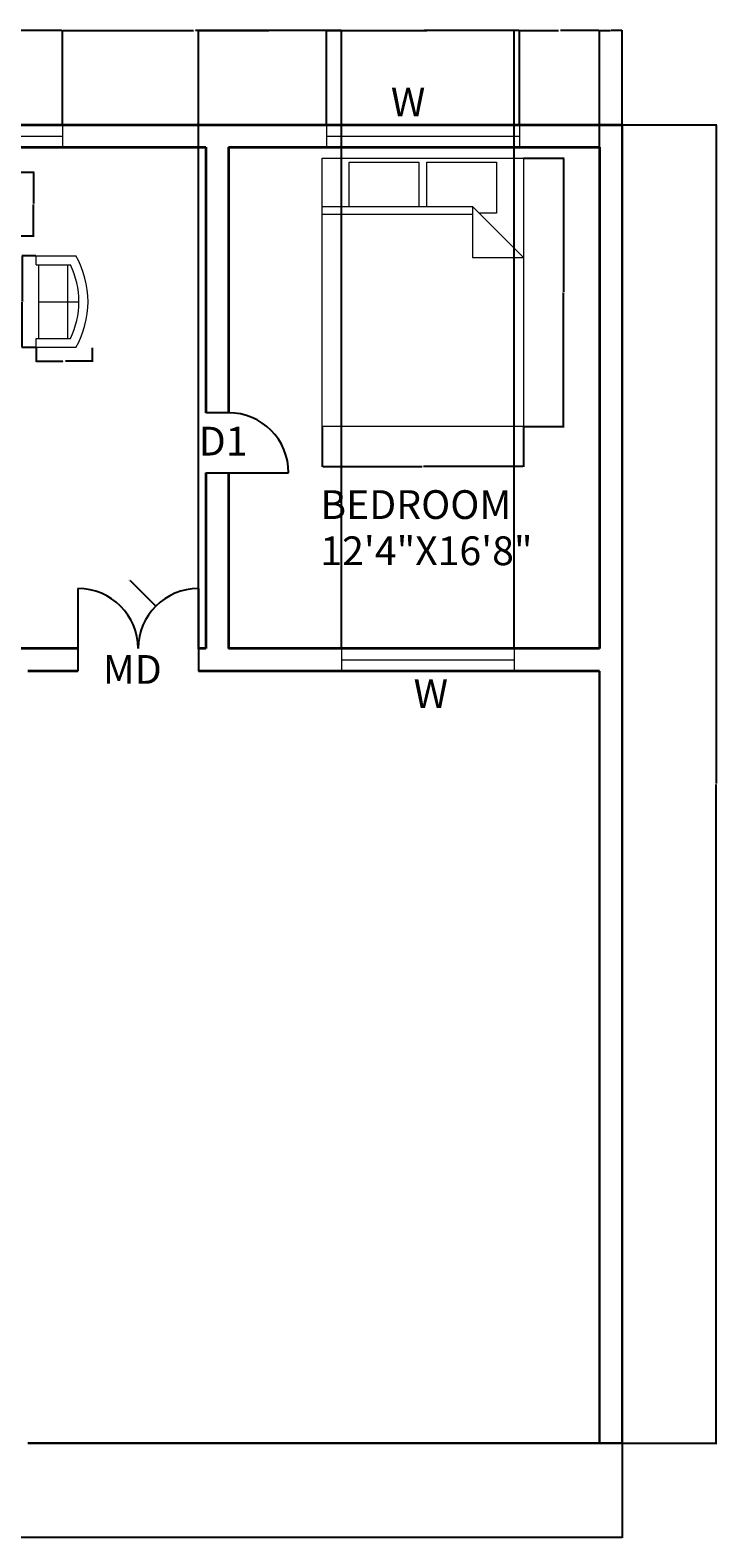
# Model space of a CAD drawing. Units: feet. Extents: x 1889 to 2708, y 1752 to 2375.
# Tile 5 of 5: x 2434 to 2708, y 1774 to 2375. Entities that reach past the tile are written whole.
import ezdxf

# ---------------------------------------------------------------- set-up
doc = ezdxf.new("R2010")
doc.units = ezdxf.units.FT
for name, color, linetype, lineweight in [('A-ANNO-DIMS', 2, 'Continuous', 18), ('A-ANNO-TEXT', 7, 'Continuous', 18), ('A-AREA-IDEN', 7, 'Continuous', 18), ('A-DOOR', 3, 'Continuous', 25), ('A-FURN', 8, 'Continuous', 18), ('A-GLAZ', 4, 'Continuous', 18), ('A-WALL', 7, 'Continuous', 35), ('C-PROP', 7, 'Continuous', 30)]:
    doc.layers.add(name, color=color, linetype=linetype, lineweight=lineweight)
doc.styles.get("Standard").update_dxf_attribs({"font": 'arial.ttf'})
doc.dimstyles.get("Standard").update_dxf_attribs({"dimtxt": 0.18, "dimasz": 0.18, "dimexe": 0.18, "dimexo": 0.0625, "dimgap": 0.09, "dimtad": 0, "dimtih": 1, "dimtoh": 1, "dimdec": 4, "dimzin": 0, "dimdsep": 46, "dimtxsty": 'Standard', "dimcen": 0.09, "dimadec": 0, "dimazin": 0, "dimtfac": 1, "dimtdec": 4, "dimtofl": 0, "dimtmove": 0, "dimatfit": 3, "dimfxl": 1, "dimtolj": 1, "dimtzin": 0, "dimarcsym": 0})

# ---------------------------------------------------------------- blocks, each defined once
blk = doc.blocks.new('Sofa - Roundback Loveseat 5 ft.')
for p, q in [((0, -32.44198), (0, -5.99998)), ((-24, -33.99998), (-24, -11.46958)), ((-23.9998, -13.38178), (23.99986, -13.38178)), ((24.00004, -33.99998), (24.00004, -11.46958)), ((-24, -32.44198), (24.00004, -32.44198))]:
    blk.add_line(p, q)
for points in [[(-24, -33.99998), (-30, -33.99998), (-30, -7.99998)], [(30.00004, -7.99998), (30.00004, -33.99998), (24.00004, -33.99998)]]:
    blk.add_lwpolyline(points)
for centre, radius, start, end in [((0, -60.24998), 60.24998, 60.13715, 119.8628), ((0, -61.38438), 55.38444, 64.32083, 115.6792)]:
    blk.add_arc(centre, radius, start, end)
blk = doc.blocks.new('Bed - Queen')
for p, q in [((0, -80.00003), (0, 0)), ((0, 0), (59.99999, 0)), ((59.99999, 0), (59.99999, -80.00003)), ((7.99999, -1.2), (28.79998, -1.2)), ((7.99999, -14.4), (7.99999, -1.2)), ((28.79998, -1.2), (28.79998, -14.4)), ((31.19999, -1.2), (51.99999, -1.2)), ((31.19999, -14.4), (31.19999, -1.2)), ((51.99999, -1.2), (51.99999, -16.4)), ((0, -14.4), (44.8, -14.4)), ((44.8, -16.8), (0, -16.8)), ((59.99999, -29.6), (44.8, -14.4)), ((44.8, -14.4), (44.8, -29.6)), ((51.99999, -16.4), (46.79936, -16.4)), ((44.8, -29.6), (59.99999, -29.6)), ((59.99999, -80.00003), (0, -80.00003))]:
    blk.add_line(p, q)
blk = doc.blocks.new('*D21')
at = {"layer": 'A-ANNO-DIMS', "color": 0, "lineweight": -2, "transparency": 16777216}
for p, q in [((2630.52, 2324.2), (2646.68, 2324.2)), ((2646.5, 2324.02), (2646.5, 2270.92)), ((2646.5, 2217.46), (2646.5, 2270.56)), ((2630.52, 2217.28), (2646.68, 2217.28))]:
    blk.add_line(p, q, dxfattribs=at)
at = {"layer": 'A-ANNO-DIMS', "color": 0, "transparency": 16777216}
for points in [[(2646.47, 2324.02), (2646.53, 2324.02), (2646.5, 2324.2)], [(2646.47, 2217.46), (2646.53, 2217.46), (2646.5, 2217.28)]]:
    blk.add_solid(points, dxfattribs=at)
at = {"layer": 'Defpoints', "color": 0, "transparency": 16777216}
for p in [(2630.46, 2324.2), (2646.5, 2324.2), (2630.46, 2217.28)]:
    blk.add_point(p, dxfattribs=at)
at = {"layer": 'A-ANNO-DIMS', "color": 0, "transparency": 16777216, "insert": (2646.5, 2270.74), "char_height": 0.18, "attachment_point": 5}
blk.add_mtext('\\A1;BED 107', dxfattribs=at)
blk = doc.blocks.new('*D22')
at = {"layer": 'A-ANNO-DIMS', "color": 0, "lineweight": -2, "transparency": 16777216}
for p, q in [((2550.26, 2217.22), (2550.26, 2201.06)), ((2630.46, 2217.22), (2630.46, 2201.06)), ((2550.44, 2201.24), (2590.14, 2201.24)), ((2630.28, 2201.24), (2590.58, 2201.24))]:
    blk.add_line(p, q, dxfattribs=at)
at = {"layer": 'A-ANNO-DIMS', "color": 0, "transparency": 16777216}
for points in [[(2550.44, 2201.27), (2550.44, 2201.21), (2550.26, 2201.24)], [(2630.28, 2201.27), (2630.28, 2201.21), (2630.46, 2201.24)]]:
    blk.add_solid(points, dxfattribs=at)
at = {"layer": 'Defpoints', "color": 0, "transparency": 16777216}
for p in [(2550.26, 2217.28), (2630.46, 2217.28), (2630.46, 2201.24)]:
    blk.add_point(p, dxfattribs=at)
at = {"layer": 'A-ANNO-DIMS', "color": 0, "transparency": 16777216, "insert": (2590.36, 2201.24), "char_height": 0.18, "attachment_point": 5}
blk.add_mtext('\\A1;80', dxfattribs=at)
blk = doc.blocks.new('*D24')
at = {"layer": 'A-ANNO-DIMS', "color": 0, "lineweight": -2, "transparency": 16777216}
for p, q in [((2426.47, 2318.69), (2435.33, 2318.69)), ((2435.15, 2318.51), (2435.15, 2306.15)), ((2435.15, 2293.42), (2435.15, 2305.78)), ((2426.47, 2293.24), (2435.33, 2293.24))]:
    blk.add_line(p, q, dxfattribs=at)
at = {"layer": 'A-ANNO-DIMS', "color": 0, "transparency": 16777216}
for points in [[(2435.12, 2318.51), (2435.18, 2318.51), (2435.15, 2318.69)], [(2435.12, 2293.42), (2435.18, 2293.42), (2435.15, 2293.24)]]:
    blk.add_solid(points, dxfattribs=at)
at = {"layer": 'Defpoints', "color": 0, "transparency": 16777216}
for p in [(2426.4, 2318.69), (2435.15, 2318.69), (2426.4, 2293.24)]:
    blk.add_point(p, dxfattribs=at)
at = {"layer": 'A-ANNO-DIMS', "color": 0, "transparency": 16777216, "insert": (2435.15, 2305.97), "char_height": 0.18, "attachment_point": 5}
blk.add_mtext('\\A1;25 TYP.', dxfattribs=at)
blk = doc.blocks.new('*D25')
at = {"layer": 'A-ANNO-DIMS', "color": 0, "lineweight": -2, "transparency": 16777216}
for p, q in [((2436.07, 2285.32), (2430.47, 2285.32)), ((2430.65, 2285.14), (2430.65, 2267.2)), ((2430.65, 2248.89), (2430.65, 2266.83)), ((2436.07, 2248.71), (2430.47, 2248.71))]:
    blk.add_line(p, q, dxfattribs=at)
at = {"layer": 'A-ANNO-DIMS', "color": 0, "transparency": 16777216}
for points in [[(2430.62, 2285.14), (2430.68, 2285.14), (2430.65, 2285.32)], [(2430.62, 2248.89), (2430.68, 2248.89), (2430.65, 2248.71)]]:
    blk.add_solid(points, dxfattribs=at)
at = {"layer": 'Defpoints', "color": 0, "transparency": 16777216}
for p in [(2436.14, 2285.32), (2430.65, 2248.71), (2436.14, 2248.71)]:
    blk.add_point(p, dxfattribs=at)
at = {"layer": 'A-ANNO-DIMS', "color": 0, "transparency": 16777216, "insert": (2430.65, 2267.01), "char_height": 0.18, "attachment_point": 5}
blk.add_mtext('\\A1;LOVESEAT 37 TYP.', dxfattribs=at)
blk = doc.blocks.new('*D26')
at = {"layer": 'A-ANNO-DIMS', "color": 0, "lineweight": -2, "transparency": 16777216}
for p, q in [((2436.14, 2248.65), (2436.14, 2243.04)), ((2458.5, 2248.65), (2458.5, 2243.04)), ((2436.32, 2243.22), (2446.79, 2243.22)), ((2458.32, 2243.22), (2447.85, 2243.22))]:
    blk.add_line(p, q, dxfattribs=at)
at = {"layer": 'A-ANNO-DIMS', "color": 0, "transparency": 16777216}
for points in [[(2436.32, 2243.25), (2436.32, 2243.19), (2436.14, 2243.22)], [(2458.32, 2243.25), (2458.32, 2243.19), (2458.5, 2243.22)]]:
    blk.add_solid(points, dxfattribs=at)
at = {"layer": 'Defpoints', "color": 0, "transparency": 16777216}
for p in [(2436.14, 2248.71), (2458.5, 2248.71), (2458.5, 2243.22)]:
    blk.add_point(p, dxfattribs=at)
at = {"layer": 'A-ANNO-DIMS', "color": 0, "transparency": 16777216, "insert": (2447.32, 2243.22), "char_height": 0.18, "attachment_point": 5}
blk.add_mtext('\\A1;22 TYP.', dxfattribs=at)
blk = doc.blocks.new('*D39')
at = {"layer": 'A-ANNO-DIMS', "color": 0, "lineweight": -2, "transparency": 16777216}
for p, q in [((2344.63, 2337.66), (2344.63, 2375.33)), ((2344.81, 2375.15), (2395.36, 2375.15)), ((2446.46, 2375.15), (2395.92, 2375.15)), ((2446.64, 2337.66), (2446.64, 2375.33))]:
    blk.add_line(p, q, dxfattribs=at)
at = {"layer": 'A-ANNO-DIMS', "color": 0, "transparency": 16777216}
for points in [[(2344.81, 2375.18), (2344.81, 2375.12), (2344.63, 2375.15)], [(2446.46, 2375.18), (2446.46, 2375.12), (2446.64, 2375.15)]]:
    blk.add_solid(points, dxfattribs=at)
at = {"layer": 'Defpoints', "color": 0, "transparency": 16777216}
for p in [(2446.64, 2375.15), (2344.63, 2337.6), (2446.64, 2337.6)]:
    blk.add_point(p, dxfattribs=at)
at = {"layer": 'A-ANNO-DIMS', "color": 0, "transparency": 16777216, "insert": (2395.64, 2375.15), "char_height": 0.18, "attachment_point": 5}
blk.add_mtext('\\A1;102', dxfattribs=at)
blk = doc.blocks.new('*D40')
at = {"layer": 'A-ANNO-DIMS', "color": 0, "lineweight": -2, "transparency": 16777216}
for p, q in [((2446.64, 2337.66), (2446.64, 2375.33)), ((2446.82, 2375.15), (2498.88, 2375.15)), ((2551.84, 2375.15), (2499.79, 2375.15)), ((2552.02, 2337.66), (2552.02, 2375.33))]:
    blk.add_line(p, q, dxfattribs=at)
at = {"layer": 'A-ANNO-DIMS', "color": 0, "transparency": 16777216}
for points in [[(2446.82, 2375.18), (2446.82, 2375.12), (2446.64, 2375.15)], [(2551.84, 2375.18), (2551.84, 2375.12), (2552.02, 2375.15)]]:
    blk.add_solid(points, dxfattribs=at)
at = {"layer": 'Defpoints', "color": 0, "transparency": 16777216}
for p in [(2552.02, 2375.15), (2446.64, 2337.6), (2552.02, 2337.6)]:
    blk.add_point(p, dxfattribs=at)
at = {"layer": 'A-ANNO-DIMS', "color": 0, "transparency": 16777216, "insert": (2499.33, 2375.15), "char_height": 0.18, "attachment_point": 5}
blk.add_mtext('\\A1;105.38', dxfattribs=at)
blk = doc.blocks.new('*D41')
at = {"layer": 'A-ANNO-DIMS', "color": 0, "lineweight": -2, "transparency": 16777216}
for p, q in [((2552.02, 2337.66), (2552.02, 2375.33)), ((2552.2, 2375.15), (2590.07, 2375.15)), ((2628.73, 2375.15), (2590.86, 2375.15)), ((2628.91, 2337.66), (2628.91, 2375.33))]:
    blk.add_line(p, q, dxfattribs=at)
at = {"layer": 'A-ANNO-DIMS', "color": 0, "transparency": 16777216}
for points in [[(2552.2, 2375.18), (2552.2, 2375.12), (2552.02, 2375.15)], [(2628.73, 2375.18), (2628.73, 2375.12), (2628.91, 2375.15)]]:
    blk.add_solid(points, dxfattribs=at)
at = {"layer": 'Defpoints', "color": 0, "transparency": 16777216}
for p in [(2628.91, 2375.15), (2552.02, 2337.6), (2628.91, 2337.6)]:
    blk.add_point(p, dxfattribs=at)
at = {"layer": 'A-ANNO-DIMS', "color": 0, "transparency": 16777216, "insert": (2590.46, 2375.15), "char_height": 0.18, "attachment_point": 5}
blk.add_mtext('\\A1;76.88', dxfattribs=at)
blk = doc.blocks.new('*D42')
at = {"layer": 'A-ANNO-DIMS', "color": 0, "lineweight": -2, "transparency": 16777216}
for p, q in [((2628.91, 2337.66), (2628.91, 2375.33)), ((2629.09, 2375.15), (2644.49, 2375.15)), ((2660.68, 2375.15), (2645.28, 2375.15)), ((2660.86, 2328.66), (2660.86, 2375.33))]:
    blk.add_line(p, q, dxfattribs=at)
at = {"layer": 'A-ANNO-DIMS', "color": 0, "transparency": 16777216}
for points in [[(2629.09, 2375.18), (2629.09, 2375.12), (2628.91, 2375.15)], [(2660.68, 2375.18), (2660.68, 2375.12), (2660.86, 2375.15)]]:
    blk.add_solid(points, dxfattribs=at)
at = {"layer": 'Defpoints', "color": 0, "transparency": 16777216}
for p in [(2660.86, 2375.15), (2628.91, 2337.6), (2660.86, 2328.6)]:
    blk.add_point(p, dxfattribs=at)
at = {"layer": 'A-ANNO-DIMS', "color": 0, "transparency": 16777216, "insert": (2644.89, 2375.15), "char_height": 0.18, "attachment_point": 5}
blk.add_mtext('\\A1;31.96', dxfattribs=at)
blk = doc.blocks.new('*D43')
at = {"layer": 'A-ANNO-DIMS', "color": 0, "lineweight": -2, "transparency": 16777216}
for p, q in [((2660.86, 2328.66), (2660.86, 2375.33)), ((2661.04, 2375.15), (2665.22, 2375.15)), ((2669.68, 2375.15), (2665.51, 2375.15)), ((2669.86, 2337.66), (2669.86, 2375.33))]:
    blk.add_line(p, q, dxfattribs=at)
at = {"layer": 'A-ANNO-DIMS', "color": 0, "transparency": 16777216}
for points in [[(2661.04, 2375.18), (2661.04, 2375.12), (2660.86, 2375.15)], [(2669.68, 2375.18), (2669.68, 2375.12), (2669.86, 2375.15)]]:
    blk.add_solid(points, dxfattribs=at)
at = {"layer": 'Defpoints', "color": 0, "transparency": 16777216}
for p in [(2669.86, 2375.15), (2669.86, 2337.6), (2660.86, 2328.6)]:
    blk.add_point(p, dxfattribs=at)
at = {"layer": 'A-ANNO-DIMS', "color": 0, "transparency": 16777216, "insert": (2665.36, 2375.15), "char_height": 0.18, "attachment_point": 5}
blk.add_mtext('\\A1;9', dxfattribs=at)
blk = doc.blocks.new('*D44')
at = {"layer": 'A-ANNO-DIMS', "color": 0, "lineweight": -2, "transparency": 16777216}
for p, q in [((1926.86, 1811.54), (1926.86, 1773.87)), ((2669.86, 1811.54), (2669.86, 1773.87)), ((1927.04, 1774.05), (2298.08, 1774.05)), ((2669.68, 1774.05), (2298.65, 1774.05))]:
    blk.add_line(p, q, dxfattribs=at)
at = {"layer": 'A-ANNO-DIMS', "color": 0, "transparency": 16777216}
for points in [[(1927.04, 1774.08), (1927.04, 1774.02), (1926.86, 1774.05)], [(2669.68, 1774.08), (2669.68, 1774.02), (2669.86, 1774.05)]]:
    blk.add_solid(points, dxfattribs=at)
at = {"layer": 'Defpoints', "color": 0, "transparency": 16777216}
for p in [(1926.86, 1811.6), (2669.86, 1811.6), (2669.86, 1774.05)]:
    blk.add_point(p, dxfattribs=at)
at = {"layer": 'A-ANNO-DIMS', "color": 0, "transparency": 16777216, "insert": (2298.36, 1774.05), "char_height": 0.18, "attachment_point": 5}
blk.add_mtext('\\A1;743', dxfattribs=at)
blk = doc.blocks.new('*D45')
at = {"layer": 'A-ANNO-DIMS', "color": 0, "lineweight": -2, "transparency": 16777216}
for p, q in [((2669.93, 2337.6), (2707.59, 2337.6)), ((2707.41, 2337.42), (2707.41, 2074.78)), ((2707.41, 1811.78), (2707.41, 2074.42)), ((2669.93, 1811.6), (2707.59, 1811.6))]:
    blk.add_line(p, q, dxfattribs=at)
at = {"layer": 'A-ANNO-DIMS', "color": 0, "transparency": 16777216}
for points in [[(2707.38, 2337.42), (2707.44, 2337.42), (2707.41, 2337.6)], [(2707.38, 1811.78), (2707.44, 1811.78), (2707.41, 1811.6)]]:
    blk.add_solid(points, dxfattribs=at)
at = {"layer": 'Defpoints', "color": 0, "transparency": 16777216}
for p in [(2669.86, 2337.6), (2707.41, 2337.6), (2669.86, 1811.6)]:
    blk.add_point(p, dxfattribs=at)
at = {"layer": 'A-ANNO-DIMS', "color": 0, "transparency": 16777216, "insert": (2707.41, 2074.6), "char_height": 0.18, "attachment_point": 5}
blk.add_mtext('\\A1;526', dxfattribs=at)
blk = doc.blocks.new('*D62')
at = {"layer": 'A-ANNO-DIMS', "color": 0, "lineweight": -2, "transparency": 16777216}
for p, q in [((2500.86, 2128.66), (2500.86, 2375.33)), ((2501.04, 2375.15), (2529.03, 2375.15)), ((2557.81, 2375.15), (2529.82, 2375.15)), ((2557.99, 2128.66), (2557.99, 2375.33))]:
    blk.add_line(p, q, dxfattribs=at)
at = {"layer": 'A-ANNO-DIMS', "color": 0, "transparency": 16777216}
for points in [[(2501.04, 2375.18), (2501.04, 2375.12), (2500.86, 2375.15)], [(2557.81, 2375.18), (2557.81, 2375.12), (2557.99, 2375.15)]]:
    blk.add_solid(points, dxfattribs=at)
at = {"layer": 'Defpoints', "color": 0, "transparency": 16777216}
for p in [(2557.99, 2375.15), (2500.86, 2128.6), (2557.99, 2128.6)]:
    blk.add_point(p, dxfattribs=at)
at = {"layer": 'A-ANNO-DIMS', "color": 0, "transparency": 16777216, "insert": (2529.43, 2375.15), "char_height": 0.18, "attachment_point": 5}
blk.add_mtext('\\A1;57.12', dxfattribs=at)
blk = doc.blocks.new('*D63')
at = {"layer": 'A-ANNO-DIMS', "color": 0, "lineweight": -2, "transparency": 16777216}
for p, q in [((2557.99, 2128.66), (2557.99, 2375.33)), ((2558.17, 2375.15), (2592.03, 2375.15)), ((2626.68, 2375.15), (2592.82, 2375.15)), ((2626.86, 2128.66), (2626.86, 2375.33))]:
    blk.add_line(p, q, dxfattribs=at)
at = {"layer": 'A-ANNO-DIMS', "color": 0, "transparency": 16777216}
for points in [[(2558.17, 2375.18), (2558.17, 2375.12), (2557.99, 2375.15)], [(2626.68, 2375.18), (2626.68, 2375.12), (2626.86, 2375.15)]]:
    blk.add_solid(points, dxfattribs=at)
at = {"layer": 'Defpoints', "color": 0, "transparency": 16777216}
for p in [(2626.86, 2375.15), (2557.99, 2128.6), (2626.86, 2128.6)]:
    blk.add_point(p, dxfattribs=at)
at = {"layer": 'A-ANNO-DIMS', "color": 0, "transparency": 16777216, "insert": (2592.42, 2375.15), "char_height": 0.18, "attachment_point": 5}
blk.add_mtext('\\A1;68.87', dxfattribs=at)
blk = doc.blocks.new('*D65')
at = {"layer": 'A-ANNO-DIMS', "color": 0, "lineweight": -2, "transparency": 16777216}
for p, q in [((2473.53, 2155.75), (2473.71, 2155.75)), ((2473.71, 2155.75), (2483.77, 2145.7)), ((2500.77, 2128.6), (2500.95, 2128.6)), ((2500.86, 2128.51), (2500.86, 2128.69))]:
    blk.add_line(p, q, dxfattribs=at)
at = {"layer": 'A-ANNO-DIMS', "color": 0, "transparency": 16777216}
blk.add_solid([(2483.79, 2145.72), (2483.75, 2145.68), (2483.89, 2145.57)], dxfattribs=at)
at = {"layer": 'Defpoints', "color": 0, "transparency": 16777216}
for p in [(2483.89, 2145.57), (2500.86, 2128.6)]:
    blk.add_point(p, dxfattribs=at)
at = {"layer": 'A-ANNO-DIMS', "color": 0, "transparency": 16777216, "insert": (2473.03, 2155.75), "char_height": 0.18, "attachment_point": 5}
blk.add_mtext('\\A1;8X R24', dxfattribs=at)

msp = doc.modelspace()

# ---------------------------------------------------------------- linework, layer by layer
at = {"layer": 'A-DOOR'}
for p, q in [((2512.8644, 2222.7086), (2503.8644, 2222.7086)), ((2503.8644, 2198.7086), (2512.8644, 2198.7086)), ((2512.8644, 2198.7086), (2536.8644, 2198.7086)), ((2452.8644, 2152.5988), (2452.8644, 2119.5988)), ((2500.8644, 2152.5988), (2500.8644, 2119.5988))]:
    msp.add_line(p, q, dxfattribs=at)
for centre, start, end in [((2512.8644, 2198.7086), 0, 90), ((2452.8644, 2128.5988), 0, 90), ((2500.8644, 2128.5988), 90, 180)]:
    msp.add_arc(centre, 24, start, end, dxfattribs=at)
at = {"layer": 'A-GLAZ'}
for p, q in [((2446.6414, 2337.5988), (2446.6414, 2328.5988)), ((2552.0213, 2337.5988), (2552.0213, 2328.5988)), ((2628.906, 2337.5988), (2628.906, 2328.5988)), ((2344.6329, 2333.0988), (2446.6414, 2333.0988)), ((2552.0213, 2333.0988), (2628.906, 2333.0988)), ((2557.9857, 2128.5988), (2557.9857, 2119.5988)), ((2557.9857, 2124.0988), (2626.8563, 2124.0988)), ((2626.8563, 2128.5988), (2626.8563, 2119.5988))]:
    msp.add_line(p, q, dxfattribs=at)
at = {"layer": 'A-WALL'}
for p, q in [((1992.8644, 2337.5988), (2669.8644, 2337.5988)), ((2279.8644, 2337.5988), (2503.8644, 2337.5988)), ((2512.8644, 2337.5988), (2669.8644, 2337.5988)), ((2279.8644, 2328.5988), (2503.8644, 2328.5988)), ((2503.8644, 2328.5988), (2503.8644, 2222.7086)), ((2512.8644, 2328.5988), (2512.8644, 2222.7086)), ((2512.8644, 2328.5988), (2660.8644, 2328.5988)), ((2660.8644, 2328.5988), (2660.8644, 2128.5988)), ((2503.8644, 2198.7086), (2503.8644, 2128.5988)), ((2512.8644, 2198.7086), (2512.8644, 2128.5988)), ((2452.8644, 2128.5988), (2390.7022, 2128.5988)), ((2503.8644, 2128.5988), (2500.8644, 2128.5988)), ((2660.8644, 2128.5988), (2512.8644, 2128.5988)), ((2452.8644, 2119.5988), (2432.8644, 2119.5988)), ((2452.8644, 2119.5988), (2432.8644, 2119.5988)), ((2503.8644, 2119.5988), (2500.8644, 2119.5988)), ((2660.8644, 2119.5988), (2500.8644, 2119.5988))]:
    msp.add_line(p, q, dxfattribs=at)
at = {"layer": 'C-PROP'}
for p, q in [((1926.8644, 2337.5988), (2669.8644, 2337.5988)), ((2669.8644, 2337.5988), (2669.8644, 1811.5988)), ((2660.8644, 2119.5988), (2660.8644, 1811.5988)), ((2432.8644, 1811.5988), (2669.8644, 1811.5988))]:
    msp.add_line(p, q, dxfattribs=at)

# ---------------------------------------------------------------- block references
at = {"layer": 'A-FURN', "xscale": 1.336562108875547, "yscale": 1.336562108875547, "zscale": 1.336562108875547}
msp.add_blockref('Bed - Queen', (2550.2627, 2324.2038), dxfattribs=at)
at = {"layer": 'A-FURN', "xscale": 0.6100416467231381, "yscale": 0.6100416467231381, "zscale": 0.6100416467231381, "rotation": 270}
msp.add_blockref('Sofa - Roundback Loveseat 5 ft.', (2456.8771, 2267.0144), dxfattribs=at)

# ---------------------------------------------------------------- texts
at = {"layer": 'A-ANNO-TEXT'}
for s, height, p in [('W', 11.4692, (2577.6297, 2340.9355)), ('D1', 11.46921, (2501.0227, 2205.6399)), ('MD', 11.46921, (2462.8076, 2114.5629)), ('W', 11.4692, (2586.6971, 2104.9075))]:
    msp.add_text(s, height=height, dxfattribs=at).set_placement(p)
at = {"layer": 'A-AREA-IDEN'}
for s, height, p in [('BEDROOM', 11.46921, (2549.5139, 2180.3279)), ('12\'4"X16\'8"', 11.469207, (2549.5139, 2161.9036))]:
    msp.add_text(s, height=height, dxfattribs=at).set_placement(p)

# ---------------------------------------------------------------- dimensions: what is measured, and where the dimension line sits
at = {"layer": 'A-ANNO-DIMS'}
for base, p1, p2, override, picture, middle in [((2446.6414, 2375.1488), (2344.6329, 2337.5988), (2446.6414, 2337.5988), {"dimdec": 0, "dimlfac": 1, "dimrnd": 0, "dimzin": 0, "dimdsep": 46, "dimlunit": 2}, '*D39', (2395.6371, 2375.1488)), ((2552.0213, 2375.1488), (2446.6414, 2337.5988), (2552.0213, 2337.5988), {"dimdec": 2, "dimlfac": 1, "dimrnd": 0, "dimzin": 0, "dimdsep": 46, "dimlunit": 2}, '*D40', (2499.3313, 2375.1488)), ((2557.9857, 2375.1488), (2500.8644, 2128.5988), (2557.9857, 2128.5988), {"dimdec": 2, "dimlfac": 1, "dimrnd": 0, "dimzin": 0, "dimdsep": 46, "dimlunit": 2}, '*D62', (2529.425, 2375.1488)), ((2628.906, 2375.1488), (2552.0213, 2337.5988), (2628.906, 2337.5988), {"dimdec": 2, "dimlfac": 1, "dimrnd": 0, "dimzin": 0, "dimdsep": 46, "dimlunit": 2}, '*D41', (2590.4637, 2375.1488)), ((2626.8563, 2375.1488), (2557.9857, 2128.5988), (2626.8563, 2128.5988), {"dimdec": 2, "dimlfac": 1, "dimrnd": 0, "dimzin": 0, "dimdsep": 46, "dimlunit": 2}, '*D63', (2592.421, 2375.1488)), ((2660.8644, 2375.1488), (2628.906, 2337.5988), (2660.8644, 2328.5988), {"dimdec": 2, "dimlfac": 1, "dimrnd": 0, "dimzin": 0, "dimdsep": 46, "dimlunit": 2}, '*D42', (2644.8852, 2375.1488)), ((2669.8644, 2375.1488), (2660.8644, 2328.5988), (2669.8644, 2337.5988), {"dimdec": 0, "dimlfac": 1, "dimrnd": 0, "dimzin": 0, "dimdsep": 46, "dimlunit": 2}, '*D43', (2665.3644, 2375.1488)), ((2630.4564, 2201.24), (2550.2627, 2217.2788), (2630.4564, 2217.2788), {"dimdec": 0, "dimlfac": 1, "dimrnd": 0, "dimzin": 0, "dimdsep": 46, "dimlunit": 2}, '*D22', (2590.3596, 2201.24)), ((2669.8644, 1774.0488), (1926.8644, 1811.5988), (2669.8644, 1811.5988), {"dimdec": 0, "dimlfac": 1, "dimrnd": 0, "dimzin": 0, "dimdsep": 46, "dimlunit": 2}, '*D44', (2298.3644, 1774.0488))]:
    dim = msp.add_linear_dim(base=base, p1=p1, p2=p2, dimstyle='Standard', override=override, dxfattribs=at)
    dim.commit()
    dim.dimension.update_dxf_attribs({"geometry": picture, "text_midpoint": middle})
dim = msp.add_linear_dim(base=(2707.4144, 2337.5988), p1=(2669.8644, 1811.5988), p2=(2669.8644, 2337.5988), angle=90, dimstyle='Standard', override={"dimdec": 0, "dimlfac": 1, "dimrnd": 0, "dimzin": 0, "dimdsep": 46, "dimlunit": 2}, dxfattribs=at)
dim.commit()
dim.dimension.update_dxf_attribs({"geometry": '*D45', "text_midpoint": (2707.4144, 2074.5988)})
for base, p1, p2, angle, text, picture, middle in [((2646.4952, 2324.2038), (2630.4564, 2217.2788), (2630.4564, 2324.2038), 90, 'BED <>', '*D21', (2646.4952, 2270.7413)), ((2435.15, 2318.6921), (2426.4042, 2293.2413), (2426.4042, 2318.6921), 90, '<> TYP.', '*D24', (2435.15, 2305.9667)), ((2430.6453, 2248.7132), (2436.1357, 2285.3157), (2436.1357, 2248.7132), 270, 'LOVESEAT <> TYP.', '*D25', (2430.6453, 2267.0144))]:
    dim = msp.add_linear_dim(base=base, p1=p1, p2=p2, angle=angle, text=text, dimstyle='Standard', override={"dimdec": 0, "dimlfac": 1, "dimrnd": 0, "dimzin": 0, "dimdsep": 46, "dimlunit": 2}, dxfattribs=at)
    dim.commit()
    dim.dimension.update_dxf_attribs({"geometry": picture, "text_midpoint": middle})
dim = msp.add_linear_dim(base=(2458.5039, 2243.2228), p1=(2436.1357, 2248.7132), p2=(2458.5039, 2248.7132), text='<> TYP.', dimstyle='Standard', override={"dimdec": 0, "dimlfac": 1, "dimrnd": 0, "dimzin": 0, "dimdsep": 46, "dimlunit": 2}, dxfattribs=at)
dim.commit()
dim.dimension.update_dxf_attribs({"geometry": '*D26', "text_midpoint": (2447.3198, 2243.2228)})
dim = msp.add_radius_dim(center=(2500.8644, 2128.5988), mpoint=(2483.8938, 2145.5692), text='8X <>', dimstyle='Standard', override={"dimdec": 0, "dimlfac": 1, "dimrnd": 0, "dimzin": 0, "dimdsep": 46, "dimlunit": 2}, dxfattribs=at)
dim.commit()
dim.dimension.update_dxf_attribs({"geometry": '*D65', "text_midpoint": (2473.0332, 2155.7515), "dimtype": 164})

doc.saveas('drawing.dxf')
